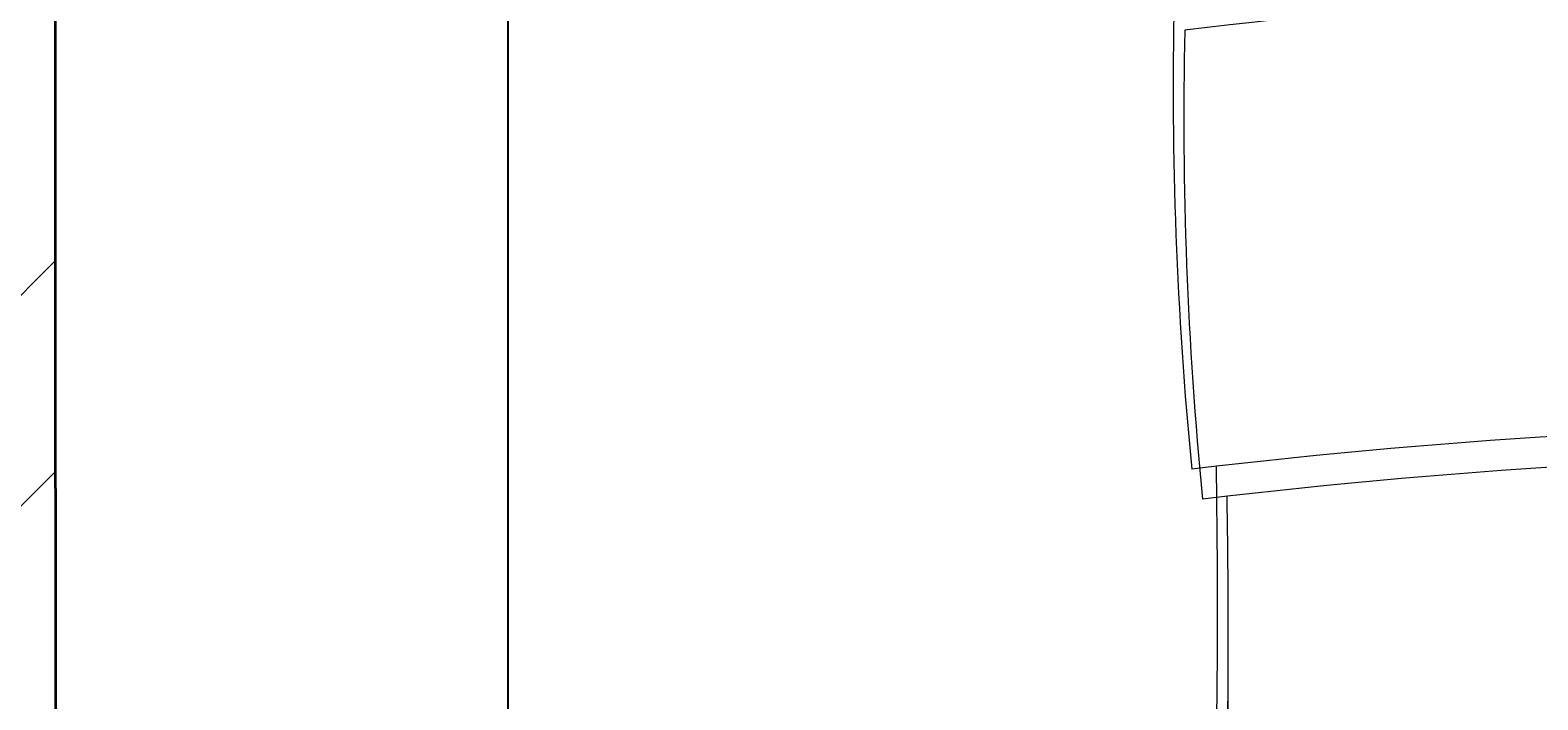
# Model space of a CAD drawing. Units: inches. Extents: x 1885 to 2748, y 783 to 2421.
# Tile 96 of 117: x 2363 to 2395, y 2314 to 2328. Entities that reach past the tile are written whole.
import ezdxf

# ---------------------------------------------------------------- set-up
doc = ezdxf.new("R2010")
doc.units = ezdxf.units.IN
for name, color, linetype, lineweight in [('A-ANNO-DIMS', 2, 'Continuous', 18), ('A-FURN', 8, 'Continuous', 13), ('A-WALL', 7, 'Continuous', 35)]:
    doc.layers.add(name, color=color, linetype=linetype, lineweight=lineweight)
doc.layers.add('A-WALL-PATT', color=85, linetype='Continuous', lineweight=13, true_color=0x58ba48)
doc.styles.get("Standard").update_dxf_attribs({"font": 'arial.ttf'})
doc.dimstyles.get("Standard").update_dxf_attribs({"dimtxt": 0.18, "dimasz": 0.18, "dimexe": 0.18, "dimexo": 0.0625, "dimgap": 0.09, "dimtad": 0, "dimtih": 1, "dimtoh": 1, "dimdec": 4, "dimzin": 0, "dimdsep": 46, "dimtxsty": 'Standard', "dimcen": 0.09, "dimadec": 0, "dimazin": 0, "dimtfac": 1, "dimtdec": 4, "dimtofl": 0, "dimtmove": 0, "dimatfit": 3, "dimfxl": 1, "dimtolj": 1, "dimtzin": 0, "dimarcsym": 0})

# ---------------------------------------------------------------- blocks, each defined once
blk = doc.blocks.new('BED-DOUBLE')
for centre, radius, start, end in [((156.959, 17.983), 129.02, 171.78449, 186.90062), ((156.959, 17.983), 129.02, 171.78449, 186.90062), ((156.32, 17.754), 129.02, 171.78449, 186.90062), ((156.32, 17.754), 129.02, 171.78449, 186.90062), ((182.695, 21.586), 164.969, 176.08655, 186.78213), ((31.817, -167.08), 170.11, 88.4762, 91.00819), ((31.817, -167.081), 170.11, 88.4762, 91.00819), ((31.177, -167.309), 170.11, 88.4762, 91.00819), ((31.177, -167.309), 170.11, 88.4762, 91.00819), ((20.1, 85.16), 83.306, 268.72178, 275.60397), ((20.1, 85.16), 83.306, 268.72178, 275.60397), ((20.739, 85.389), 83.306, 268.72178, 275.60397), ((20.739, 85.389), 83.306, 268.72178, 275.60397)]:
    blk.add_arc(centre, radius, start, end)
blk = doc.blocks.new('*D27')
at = {"layer": 'A-ANNO-DIMS', "color": 0, "lineweight": -2, "transparency": 16777216}
for p, q in [((2385.079, 2346.649), (2372.729, 2346.649)), ((2372.909, 2346.469), (2372.909, 2306.056)), ((2372.909, 2265.28), (2372.909, 2305.693)), ((2385.079, 2265.1), (2372.729, 2265.1))]:
    blk.add_line(p, q, dxfattribs=at)
at = {"layer": 'A-ANNO-DIMS', "color": 0, "transparency": 16777216}
for points in [[(2372.879, 2346.469), (2372.939, 2346.469), (2372.909, 2346.649)], [(2372.879, 2265.28), (2372.939, 2265.28), (2372.909, 2265.1)]]:
    blk.add_solid(points, dxfattribs=at)
at = {"layer": 'Defpoints', "color": 0, "transparency": 16777216}
for p in [(2385.141, 2346.649), (2372.909, 2265.1), (2385.141, 2265.1)]:
    blk.add_point(p, dxfattribs=at)
at = {"layer": 'A-ANNO-DIMS', "color": 0, "transparency": 16777216, "insert": (2372.909, 2305.874), "char_height": 0.18, "attachment_point": 5}
blk.add_mtext('\\A1;BED 82 TYP.', dxfattribs=at)

msp = doc.modelspace()

# ---------------------------------------------------------------- hatches: boundary and pattern name
at = {"layer": 'A-WALL-PATT'}
h = msp.add_hatch(dxfattribs=at)
h.set_pattern_fill('ANSI32', color=256)
h.paths.add_polyline_path([(2007.772, 2318.006), (1980.774, 2318.006), (1980.774, 2281.215), (1985.274, 2281.215), (1985.274, 2313.506), (2007.772, 2313.506), (2007.772, 2315.756)])
h.paths.add_polyline_path([(2094.324, 2318.006), (2067.772, 2318.006), (2067.772, 2313.506), (2094.324, 2313.506), (2094.324, 2315.756)])
h.paths.add_polyline_path([(2131.367, 2315.756), (2131.367, 2318.006), (2131.189, 2318.006), (2112.609, 2318.006), (2112.609, 2313.506), (2117.274, 2313.506), (2117.274, 2255.201), (2121.774, 2255.201), (2121.774, 2313.506), (2131.367, 2313.506)])
h.paths.add_polyline_path([(2190.512, 2318.006), (2155.367, 2318.006), (2155.367, 2313.506), (2169.774, 2313.506), (2169.774, 2229.506), (2121.774, 2229.506), (2121.774, 2233.451), (2119.524, 2233.451), (2117.274, 2233.451), (2117.274, 2201.101), (2121.774, 2201.101), (2121.774, 2225.006), (2169.774, 2225.006), (2169.774, 2165.006), (2306.274, 2165.006), (2306.274, 2066.006), (2310.774, 2066.006), (2344.274, 2066.006), (2486.274, 2066.006), (2486.274, 1886.006), (2483.02, 1886.006), (2483.02, 1881.506), (2486.274, 1881.506), (2486.274, 1880.678), (2490.774, 1880.678), (2490.774, 2070.506), (2344.274, 2070.506), (2310.774, 2070.506), (2310.774, 2165.006), (2310.774, 2173.636), (2308.524, 2173.636), (2306.274, 2173.636), (2306.274, 2169.506), (2174.274, 2169.506), (2174.274, 2313.506), (2190.512, 2313.506), (2190.512, 2315.756)])
h.paths.add_polyline_path([(1985.274, 2221.215), (1980.774, 2221.215), (1980.774, 2165.006), (1992.774, 2165.006), (1992.774, 2141.927), (1997.274, 2141.927), (1997.274, 2165.006), (2117.274, 2165.006), (2117.274, 2163.126), (2121.774, 2163.126), (2121.774, 2172.734), (2119.524, 2172.734), (2117.274, 2172.734), (2117.274, 2169.506), (1985.274, 2169.506)])
h.paths.add_polyline_path([(1997.274, 2105.927), (1992.774, 2105.927), (1992.774, 2070.506), (2016.774, 2070.506), (2016.774, 2059.123), (2019.024, 2059.123), (2021.274, 2059.123), (2021.274, 2070.506), (2117.274, 2070.506), (2117.274, 2022.506), (2114.423, 2022.506), (2114.423, 2018.006), (2123.627, 2018.006), (2123.627, 2020.256), (2123.627, 2022.506), (2121.774, 2022.506), (2121.774, 2142.587), (2119.524, 2142.587), (2117.274, 2142.587), (2117.274, 2075.006), (1997.274, 2075.006)])
h.paths.add_polyline_path([(2092.029, 2020.256), (2092.029, 2022.506), (2021.274, 2022.506), (2021.274, 2035.123), (2016.774, 2035.123), (2016.774, 2018.006), (2016.774, 1978.784), (2021.274, 1978.784), (2021.274, 2018.006), (2092.029, 2018.006)])
h.paths.add_polyline_path([(2260.938, 2022.506), (2153.105, 2022.506), (2153.105, 2020.256), (2153.105, 2018.006), (2155.274, 2018.006), (2155.274, 1886.006), (2107.629, 1886.006), (2107.629, 1881.506), (2182.911, 1881.506), (2182.911, 1883.756), (2182.911, 1886.006), (2159.774, 1886.006), (2159.774, 2018.006), (2260.938, 2018.006), (2260.938, 2020.256)])
h.paths.add_polyline_path([(2047.629, 1883.756), (2047.629, 1886.006), (2021.274, 1886.006), (2021.274, 1918.784), (2019.024, 1918.784), (2016.774, 1918.784), (2016.774, 1881.506), (2047.629, 1881.506)])
h.paths.add_polyline_path([(2306.361, 1883.756), (2306.361, 1886.006), (2296.274, 1886.006), (2296.274, 1982.006), (2316.535, 1982.006), (2316.535, 1984.256), (2316.535, 1986.506), (2296.274, 1986.506), (2296.274, 2022.506), (2289.276, 2022.506), (2289.276, 2018.006), (2291.774, 2018.006), (2291.774, 1886.006), (2242.911, 1886.006), (2242.911, 1881.506), (2306.361, 1881.506)], flags=17)
h.paths.add_polyline_path([(1985.274, 1843.006), (2021.6, 1843.006), (2021.534, 1845.441), (2021.477, 1847.506), (1980.774, 1847.506), (1980.774, 1809.446), (1985.274, 1809.446)])
h.paths.add_polyline_path([(2131.482, 1845.256), (2131.482, 1847.506), (2081.534, 1847.506), (2081.534, 1843.006), (2117.274, 1843.006), (2117.274, 1784.147), (2119.524, 1784.147), (2121.774, 1784.147), (2121.774, 1843.006), (2131.482, 1843.006)])
h.paths.add_polyline_path([(2203.886, 1847.506), (2155.482, 1847.506), (2155.482, 1843.006), (2169.774, 1843.006), (2169.774, 1759.006), (2121.774, 1759.006), (2121.774, 1761.457), (2117.274, 1761.457), (2117.274, 1730.429), (2121.774, 1730.429), (2121.774, 1754.506), (2177.421, 1754.506), (2177.421, 1756.756), (2177.421, 1759.006), (2174.274, 1759.006), (2174.274, 1843.006), (2203.886, 1843.006)])
h.paths.add_polyline_path([(2335.554, 1845.256), (2335.554, 1847.506), (2239.886, 1847.506), (2239.886, 1843.006), (2306.274, 1843.006), (2306.274, 1759.006), (2199.486, 1759.006), (2199.486, 1754.506), (2310.774, 1754.506), (2310.774, 1843.006), (2335.554, 1843.006)])
h.paths.add_polyline_path([(2348.774, 2022.506), (2344.274, 2022.506), (2344.274, 1986.506), (2341.681, 1986.506), (2341.681, 1982.006), (2344.274, 1982.006), (2344.274, 1886.006), (2330.361, 1886.006), (2330.361, 1881.506), (2361.627, 1881.506), (2361.627, 1883.756), (2361.627, 1886.006), (2348.774, 1886.006)], flags=17)
h.paths.add_polyline_path([(2283.251, 2315.756), (2283.251, 2318.006), (2238.512, 2318.006), (2238.512, 2313.506), (2283.251, 2313.506)], flags=17)
h.paths.add_polyline_path([(2363.274, 2348.006), (2388.677, 2348.006), (2388.677, 2350.256), (2388.677, 2352.506), (2358.774, 2352.506), (2358.774, 2348.006), (2358.774, 2318.006), (2344.481, 2318.006), (2344.481, 2313.506), (2358.774, 2313.506), (2358.774, 2229.506), (2310.774, 2229.506), (2310.774, 2231.952), (2306.274, 2231.952), (2306.274, 2205.611), (2310.774, 2205.611), (2310.774, 2225.006), (2358.774, 2225.006), (2358.774, 2211.506), (2452.329, 2211.506), (2452.329, 2213.756), (2452.329, 2216.006), (2363.274, 2216.006), (2363.274, 2318.006)])
h.paths.add_polyline_path([(2310.774, 2313.506), (2320.481, 2313.506), (2320.481, 2315.756), (2320.481, 2318.006), (2302.728, 2318.006), (2302.728, 2313.506), (2306.274, 2313.506), (2306.274, 2251.076), (2310.774, 2251.076)], flags=17)
h.paths.add_polyline_path([(2490.774, 2352.506), (2486.274, 2352.506), (2448.677, 2352.506), (2448.677, 2348.006), (2486.274, 2348.006), (2486.274, 2318.006), (2486.274, 2216.006), (2481.78, 2216.006), (2481.78, 2211.506), (2486.274, 2211.506), (2486.274, 2165.006), (2493.289, 2165.006), (2493.289, 2167.256), (2493.289, 2169.506), (2490.774, 2169.506), (2490.774, 2313.506), (2494.429, 2313.506), (2494.429, 2318.006), (2490.774, 2318.006)])
h.paths.add_polyline_path([(2534.653, 2318.006), (2515.691, 2318.006), (2515.691, 2313.506), (2534.653, 2313.506), (2534.653, 2315.756)])
h.paths.add_polyline_path([(2618.274, 2318.006), (2594.653, 2318.006), (2594.653, 2313.506), (2613.774, 2313.506), (2613.774, 2281.706), (2618.274, 2281.706)])
h.paths.add_polyline_path([(2618.274, 2221.706), (2613.774, 2221.706), (2613.774, 2169.506), (2554.019, 2169.506), (2554.019, 2165.006), (2613.774, 2165.006), (2613.774, 2152.878), (2618.274, 2152.878)])
h.paths.add_polyline_path([(2618.274, 2128.878), (2616.024, 2128.878), (2613.774, 2128.878), (2613.774, 2117.006), (2529.774, 2117.006), (2529.774, 2165.006), (2532.848, 2165.006), (2532.848, 2169.506), (2522.867, 2169.506), (2522.867, 2165.006), (2525.274, 2165.006), (2525.274, 2117.006), (2525.274, 2112.506), (2525.274, 2108.576), (2529.774, 2108.576), (2529.774, 2112.506), (2613.774, 2112.506), (2613.774, 2080.19), (2618.274, 2080.19)])
h.paths.add_polyline_path([(2618.274, 2044.19), (2616.024, 2044.19), (2613.774, 2044.19), (2613.774, 2015.506), (2529.774, 2015.506), (2529.774, 2088.582), (2527.524, 2088.582), (2525.274, 2088.582), (2525.274, 2011.006), (2613.774, 2011.006), (2613.774, 1956.755), (2618.274, 1956.755)])
h.paths.add_polyline_path([(2618.274, 1881.506), (2618.274, 1896.755), (2613.774, 1896.755), (2613.774, 1881.506), (2613.774, 1847.506), (2592.715, 1847.506), (2592.715, 1843.006), (2613.774, 1843.006), (2613.774, 1765.006), (2613.774, 1760.506), (2609.621, 1760.506), (2609.621, 1756.006), (2613.774, 1756.006), (2613.774, 1660.006), (2608.544, 1660.006), (2608.544, 1655.506), (2613.774, 1655.506), (2613.774, 1508.158), (2618.274, 1508.158)])
h.paths.add_polyline_path([(2565.774, 1843.006), (2568.997, 1843.006), (2568.997, 1847.506), (2490.774, 1847.506), (2490.774, 1849.7), (2488.524, 1849.7), (2486.274, 1849.7), (2486.274, 1847.506), (2477.274, 1847.506), (2477.274, 1838.506), (2477.274, 1821.493), (2486.274, 1821.493), (2486.274, 1838.506), (2561.274, 1838.506), (2561.274, 1765.006), (2486.274, 1765.006), (2486.274, 1786.157), (2477.274, 1786.157), (2477.274, 1765.006), (2477.274, 1756.006), (2486.274, 1756.006), (2565.774, 1756.006), (2585.621, 1756.006), (2585.621, 1758.256), (2585.621, 1760.506), (2565.774, 1760.506), (2565.774, 1765.006)])
h.paths.add_polyline_path([(2486.274, 1651.006), (2561.274, 1651.006), (2561.274, 1567.006), (2486.274, 1567.006), (2486.274, 1591.321), (2477.274, 1591.321), (2477.274, 1567.006), (2477.274, 1558.006), (2477.274, 1555.439), (2481.774, 1555.439), (2481.774, 1558.006), (2568.653, 1558.006), (2568.653, 1560.256), (2568.653, 1562.506), (2565.774, 1562.506), (2565.774, 1655.506), (2584.544, 1655.506), (2584.544, 1657.756), (2584.544, 1660.006), (2565.774, 1660.006), (2486.274, 1660.006), (2477.274, 1660.006), (2477.274, 1651.006), (2477.274, 1632.989), (2486.274, 1632.989)])
h.paths.add_polyline_path([(2449.967, 1883.756), (2449.967, 1886.006), (2421.627, 1886.006), (2421.627, 1881.506), (2449.967, 1881.506)], flags=17)
h.paths.add_polyline_path([(2447.274, 1847.506), (2395.554, 1847.506), (2395.554, 1843.006), (2442.774, 1843.006), (2442.774, 1809.27), (2447.274, 1809.27)])
h.paths.add_polyline_path([(1985.274, 1749.446), (1980.774, 1749.446), (1980.774, 1694.504), (1985.274, 1694.504), (1985.274, 1694.506), (1986.897, 1694.506), (1986.897, 1697.78), (1986.897, 1699.006), (1985.274, 1699.006)])
h.paths.add_polyline_path([(2152.774, 1699.006), (2121.774, 1699.006), (2121.774, 1703.668), (2119.524, 1703.668), (2117.274, 1703.668), (2117.274, 1699.006), (2009.219, 1699.006), (2009.219, 1694.506), (2148.274, 1694.506), (2148.274, 1692.631), (2152.774, 1692.631)])
h.paths.add_polyline_path([(2016.274, 1694.506), (2011.774, 1694.506), (2011.774, 1558.006), (2040.806, 1558.006), (2040.806, 1560.256), (2040.806, 1562.506), (2016.274, 1562.506)])
h.paths.add_polyline_path([(2152.774, 1663.017), (2150.524, 1663.017), (2148.274, 1663.017), (2148.274, 1562.506), (2100.806, 1562.506), (2100.806, 1558.006), (2165.119, 1558.006), (2165.119, 1560.256), (2165.119, 1562.506), (2152.774, 1562.506), (2152.774, 1610.506), (2224.774, 1610.506), (2224.774, 1607.99), (2229.274, 1607.99), (2229.274, 1615.006), (2152.774, 1615.006)])
h.paths.add_polyline_path([(2238.613, 1560.256), (2238.613, 1562.506), (2229.274, 1562.506), (2229.274, 1588.756), (2227.024, 1588.763), (2224.774, 1588.771), (2224.774, 1562.506), (2189.119, 1562.506), (2189.119, 1558.006), (2238.613, 1558.006)])
h.paths.add_polyline_path([(2336.024, 1560.256), (2336.024, 1562.506), (2310.774, 1562.506), (2310.774, 1656.347), (2308.524, 1656.347), (2306.274, 1656.347), (2306.274, 1562.506), (2286.613, 1562.506), (2286.613, 1558.006), (2336.024, 1558.006)])
h.paths.add_polyline_path([(2447.274, 1690.968), (2445.024, 1690.968), (2442.774, 1690.968), (2442.774, 1687.006), (2306.274, 1687.006), (2306.274, 1680.75), (2310.774, 1680.75), (2310.774, 1682.506), (2442.774, 1682.506), (2442.774, 1562.506), (2396.024, 1562.506), (2396.024, 1558.006), (2447.274, 1558.006)])
h.paths.add_polyline_path([(2447.274, 1749.27), (2445.024, 1749.27), (2442.774, 1749.27), (2442.774, 1717.232), (2447.274, 1717.232)])
h.paths.add_polyline_path([(2044.674, 1521.756), (2044.674, 1524.006), (2007.274, 1524.006), (2007.274, 1503.49), (2009.524, 1503.49), (2011.774, 1503.49), (2011.774, 1519.506), (2044.674, 1519.506)])
h.paths.add_polyline_path([(2177.969, 1521.756), (2177.969, 1524.006), (2104.674, 1524.006), (2104.674, 1519.506), (2145.774, 1519.506), (2145.774, 1387.506), (2143.37, 1387.506), (2143.37, 1383.006), (2251.585, 1383.006), (2251.585, 1385.256), (2251.585, 1387.506), (2150.274, 1387.506), (2150.274, 1519.506), (2177.969, 1519.506)])
h.paths.add_polyline_path([(2298.704, 1524.006), (2237.969, 1524.006), (2237.969, 1519.506), (2282.274, 1519.506), (2282.274, 1387.506), (2279.683, 1387.506), (2279.683, 1383.006), (2286.774, 1383.006), (2286.774, 1419.006), (2312.451, 1419.006), (2312.451, 1421.256), (2312.451, 1423.506), (2286.774, 1423.506), (2286.774, 1519.506), (2298.704, 1519.506), (2298.704, 1521.722)], flags=17)
h.paths.add_polyline_path([(2361.897, 1521.756), (2361.897, 1524.006), (2322.704, 1524.006), (2322.704, 1519.506), (2334.774, 1519.506), (2334.774, 1423.506), (2331.93, 1423.506), (2331.93, 1419.006), (2334.774, 1419.006), (2334.774, 1387.506), (2334.774, 1383.228), (2339.274, 1383.228), (2339.274, 1387.506), (2339.274, 1519.506), (2361.897, 1519.506)], flags=17)
h.paths.add_polyline_path([(2447.274, 1521.756), (2447.274, 1524.006), (2421.897, 1524.006), (2421.897, 1519.506), (2447.274, 1519.506)], flags=17)
h.paths.add_polyline_path([(2481.774, 1529.6), (2479.524, 1529.6), (2477.274, 1529.6), (2477.274, 1524.006), (2474.489, 1524.006), (2474.489, 1519.506), (2477.274, 1519.506), (2477.274, 1334.506), (2296.774, 1334.506), (2296.774, 1240.506), (2160.274, 1240.506), (2160.274, 1180.506), (2112.274, 1180.506), (2112.274, 1207.692), (2110.024, 1207.692), (2107.774, 1207.692), (2107.774, 1171.609), (2112.274, 1171.609), (2112.274, 1176.006), (2160.274, 1176.006), (2160.274, 1092.006), (2144.221, 1092.006), (2144.221, 1087.506), (2189.497, 1087.506), (2189.497, 1089.756), (2189.497, 1092.006), (2164.774, 1092.006), (2164.774, 1236.006), (2296.774, 1236.006), (2296.774, 1231.912), (2301.274, 1231.912), (2301.274, 1330.006), (2481.774, 1330.006), (2481.774, 1387.506)])
h.paths.add_polyline_path([(2618.274, 1448.158), (2613.774, 1448.158), (2613.774, 1382.506), (2529.774, 1382.506), (2525.274, 1382.506), (2525.274, 1307.062), (2529.774, 1307.062), (2529.774, 1378.006), (2613.774, 1378.006), (2613.774, 1354.988), (2618.274, 1354.988)])
h.paths.add_polyline_path([(2618.274, 1318.988), (2613.774, 1318.988), (2613.774, 1281.006), (2529.774, 1281.006), (2529.774, 1283.786), (2527.524, 1283.786), (2525.274, 1283.786), (2525.274, 1228.506), (2516.794, 1228.506), (2516.794, 1224.006), (2533.484, 1224.006), (2533.484, 1226.256), (2533.484, 1228.506), (2529.774, 1228.506), (2529.774, 1276.506), (2613.774, 1276.506), (2613.774, 1266.02), (2618.274, 1266.02)])
h.paths.add_polyline_path([(2618.274, 1134.964), (2613.774, 1134.964), (2613.774, 1092.006), (2594.545, 1092.006), (2594.545, 1087.506), (2618.274, 1087.506)])
h.paths.add_polyline_path([(2534.545, 1092.006), (2509.765, 1092.006), (2509.765, 1087.506), (2534.545, 1087.506), (2534.545, 1089.756)])
h.paths.add_polyline_path([(2481.274, 1224.006), (2484.117, 1224.006), (2484.117, 1226.256), (2484.117, 1228.506), (2476.774, 1228.506), (2476.774, 1198.506), (2471.61, 1198.506), (2471.61, 1194.006), (2476.774, 1194.006), (2476.774, 1062.006), (2436.894, 1062.006), (2436.894, 1057.506), (2476.774, 1057.506), (2481.274, 1057.506), (2481.274, 1062.006), (2481.274, 1087.506), (2485.354, 1087.506), (2485.354, 1089.756), (2485.354, 1092.006), (2481.274, 1092.006), (2481.274, 1117.506)])
h.paths.add_polyline_path([(2439.898, 1198.506), (2349.274, 1198.506), (2349.274, 1194.006), (2349.274, 1180.506), (2301.274, 1180.506), (2301.274, 1201.896), (2299.024, 1201.896), (2296.774, 1201.896), (2296.774, 1172.335), (2299.024, 1172.335), (2301.274, 1172.335), (2301.274, 1176.006), (2349.274, 1176.006), (2349.274, 1092.006), (2334.452, 1092.006), (2334.452, 1087.506), (2349.274, 1087.506), (2349.274, 1057.506), (2353.774, 1057.506), (2376.894, 1057.506), (2376.894, 1059.756), (2376.894, 1062.006), (2353.774, 1062.006), (2353.774, 1087.506), (2353.774, 1180.506), (2353.774, 1194.006), (2439.898, 1194.006), (2439.898, 1196.256)])
h.paths.add_polyline_path([(2270.596, 1089.756), (2270.596, 1092.006), (2249.497, 1092.006), (2249.497, 1087.506), (2270.596, 1087.506)], flags=17)
h.paths.add_polyline_path([(2310.452, 1092.006), (2301.274, 1092.006), (2301.274, 1153.292), (2296.774, 1153.292), (2296.774, 1092.006), (2293.786, 1092.006), (2293.786, 1087.506), (2310.452, 1087.506), (2310.452, 1089.756)], flags=17)
h.paths.add_polyline_path([(2112.274, 1150.328), (2110.024, 1150.328), (2107.774, 1150.328), (2107.774, 1092.006), (2104.465, 1092.006), (2104.465, 1087.506), (2120.221, 1087.506), (2120.221, 1089.756), (2120.221, 1092.006), (2112.274, 1092.006)])
h.paths.add_polyline_path([(2082.172, 1092.006), (2058.144, 1092.006), (2058.144, 1087.506), (2082.172, 1087.506), (2082.172, 1089.756)])
h.paths.add_polyline_path([(1975.774, 1145.638), (1971.274, 1145.638), (1971.274, 1087.506), (1980.774, 1087.506), (1998.144, 1087.506), (1998.144, 1089.756), (1998.144, 1092.006), (1985.274, 1092.006), (1975.774, 1092.006)])
h.paths.add_polyline_path([(2112.274, 1244.385), (2110.024, 1244.385), (2107.774, 1244.385), (2107.774, 1240.506), (1992.274, 1240.506), (1992.274, 1271.008), (1987.774, 1271.008), (1987.774, 1240.506), (1980.774, 1240.506), (1975.774, 1240.506), (1971.274, 1240.506), (1971.274, 1205.638), (1975.774, 1205.638), (1975.774, 1236.006), (2107.774, 1236.006), (2107.774, 1233.444), (2112.274, 1233.444), (2112.274, 1236.006)])
h.paths.add_polyline_path([(2112.274, 1383.006), (2114.783, 1383.006), (2114.783, 1385.256), (2114.783, 1387.506), (2102.476, 1387.506), (2102.476, 1383.006), (2107.774, 1383.006), (2107.774, 1335.006), (2011.774, 1335.006), (2011.774, 1349.939), (2007.274, 1349.939), (2007.274, 1335.006), (1987.774, 1335.006), (1987.774, 1330.506), (1987.774, 1307.008), (1992.274, 1307.008), (1992.274, 1330.506), (2007.274, 1330.506), (2107.774, 1330.506), (2107.774, 1264.711), (2112.274, 1264.711)])
h.paths.add_polyline_path([(2077.857, 1387.506), (2011.774, 1387.506), (2011.774, 1390.036), (2009.524, 1390.036), (2007.274, 1390.036), (2007.274, 1373.939), (2011.774, 1373.939), (2011.774, 1383.006), (2077.857, 1383.006)])
h.paths.add_polyline_path([(2011.774, 1443.49), (2007.274, 1443.49), (2007.274, 1410.248), (2011.774, 1410.248)])

# ---------------------------------------------------------------- linework, layer by layer
at = {"layer": 'A-WALL'}
for q in [(2363.274, 2348.006), (2363.274, 2216.006)]:
    msp.add_line((2363.274, 2318.006), q, dxfattribs=at)

# ---------------------------------------------------------------- block references
at = {"layer": 'A-FURN', "rotation": 269.9999998331857}
msp.add_blockref('BED-DOUBLE', (2385.229, 2346.652), dxfattribs=at)

# ---------------------------------------------------------------- dimensions: what is measured, and where the dimension line sits
at = {"layer": 'A-ANNO-DIMS'}
dim = msp.add_linear_dim(base=(2372.909, 2265.1), p1=(2385.141, 2346.649), p2=(2385.141, 2265.1), angle=270, text='BED <> TYP.', dimstyle='Standard', override={"dimdec": 0, "dimlfac": 1, "dimrnd": 0, "dimzin": 0, "dimdsep": 46, "dimlunit": 2}, dxfattribs=at)
dim.commit()
dim.dimension.update_dxf_attribs({"geometry": '*D27', "text_midpoint": (2372.909, 2305.874)})

doc.saveas('drawing.dxf')
